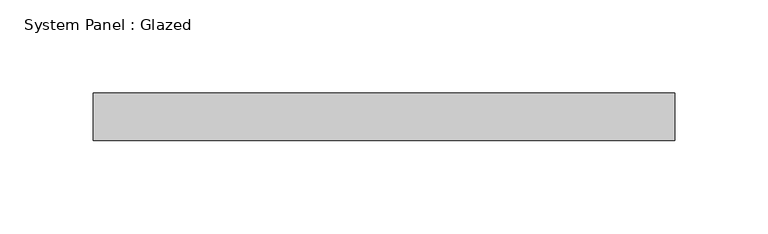
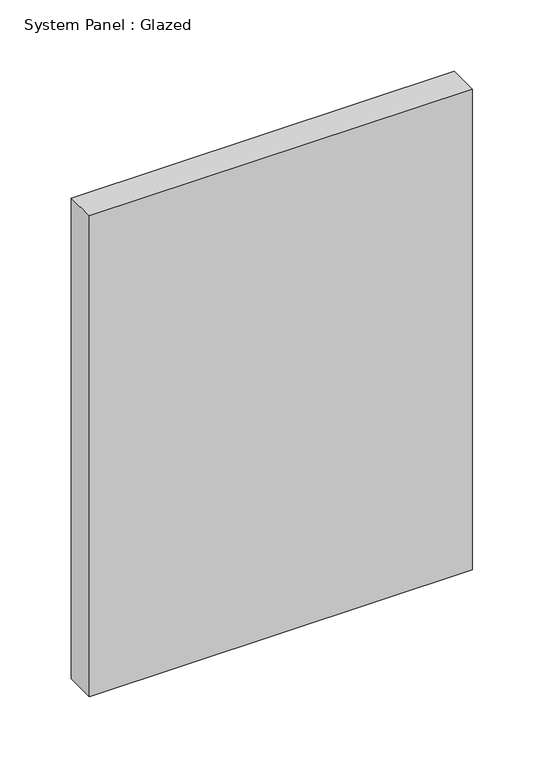
"""IFC4 building model written with IfcOpenShell, lengths in millimetres: plate geometry, System Panel : Glazed."""

from ifc_helpers import new_model, si_unit, origin, origin_with_axes, place, context, project, spatial, polyline, outline, extrude, source, transform, mapped, element, save


def system_panel_glazed_bc497e33(model_context):
    return source(origin(), model_context, "Body", "SweptSolid", [
        extrude(outline(polyline([(155.575, 19.05), (-155.575, 19.05), (-155.575, 44.45), (155.575, 44.45), (155.575, 19.05)])), origin_with_axes(), (0.0, 0.0, 1.0), 412.75),
    ])


if __name__ == "__main__":
    model = new_model("IFC4")
    model_context = context("Model", 3, world=origin())
    ifc_project = project(units=[si_unit("LENGTHUNIT", "METRE", prefix="MILLI")], contexts=[model_context])
    site = spatial("IfcSite", under=ifc_project)
    building = spatial("IfcBuilding", under=site)
    placement = place(None, origin())
    system_panel_glazed_shape = system_panel_glazed_bc497e33(model_context)
    element("IfcPlate", 1, ObjectType="System Panel : Glazed", at=placement, inside=building, context=model_context, shape_type="MappedRepresentation", body=[
        mapped(system_panel_glazed_shape, transform((0.0, 0.0, 0.0), x_axis=(1.0, 0.0, 0.0), y_axis=(0.0, 1.0, 0.0), z_axis=(0.0, 0.0, 1.0))),
    ])
    save(model, "model.ifc")

# Revit data of these elements
# Type "System Panel : Glazed"
#   Construction Type Id = "GSP4R"
#   Analytic Construction = "1/8 in Pilkington single glazing"
#   Visual Light Transmittance = 0.9
#   Solar Heat Gain Coefficient = 0.86
#   Heat Transfer Coefficient (U) = 1.18115 BTU/(h·ft²·°F)
#   Define Thermal Properties by = 1
# Element 1 (IfcPlate, "System Panel : Glazed")
#   Materials on its faces: "Glass"
# Materials
#   "Glass": class "Glass", colour RGB 0 128 192, transparency 0.75, Description = "Soda Lime Glass", Cost = 0
